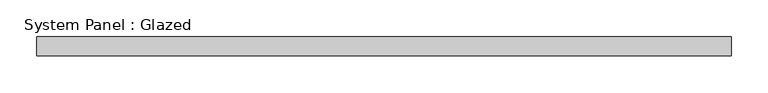
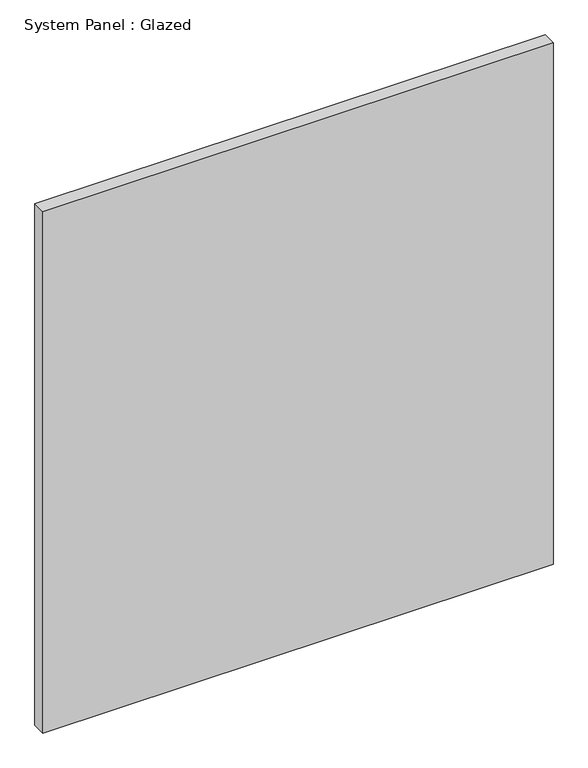
"""IFC4 building model written with IfcOpenShell, lengths in millimetres: plate geometry, System Panel : Glazed."""

from ifc_helpers import new_model, si_unit, origin, origin_with_axes, place, context, project, spatial, polyline, outline, extrude, source, transform, mapped, element, save


def system_panel_glazed_0610b94e(model_context):
    return source(origin(), model_context, "Body", "SweptSolid", [
        extrude(outline(polyline([(469.9, 19.05), (-469.9, 19.05), (-469.9, 44.45), (469.9, 44.45), (469.9, 19.05)])), origin_with_axes(), (0.0, 0.0, 1.0), 1015.3491558),
    ])


if __name__ == "__main__":
    model = new_model("IFC4")
    model_context = context("Model", 3, world=origin())
    ifc_project = project(units=[si_unit("LENGTHUNIT", "METRE", prefix="MILLI")], contexts=[model_context])
    site = spatial("IfcSite", under=ifc_project)
    building = spatial("IfcBuilding", under=site)
    placement = place(None, origin())
    system_panel_glazed_shape = system_panel_glazed_0610b94e(model_context)
    element("IfcPlate", 1, ObjectType="System Panel : Glazed", at=placement, inside=building, context=model_context, shape_type="MappedRepresentation", body=[
        mapped(system_panel_glazed_shape, transform((0.0, 0.0, 0.0), x_axis=(1.0, 0.0, 0.0), y_axis=(0.0, 1.0, 0.0), z_axis=(0.0, 0.0, 1.0))),
    ])
    save(model, "model.ifc")

# Revit data of these elements
# Type "System Panel : Glazed"
#   Construction Type Id = "GSP4R"
#   Analytic Construction = "1/8 in Pilkington single glazing"
#   Visual Light Transmittance = 0.9
#   Solar Heat Gain Coefficient = 0.86
#   Heat Transfer Coefficient (U) = 1.18115 BTU/(h·ft²·°F)
#   Define Thermal Properties by = 1
# Element 1 (IfcPlate, "System Panel : Glazed")
#   Materials on its faces: "Glass"
# Materials
#   "Glass": class "Glass", colour RGB 0 128 192, transparency 0.75, Description = "Soda Lime Glass", Cost = 0
